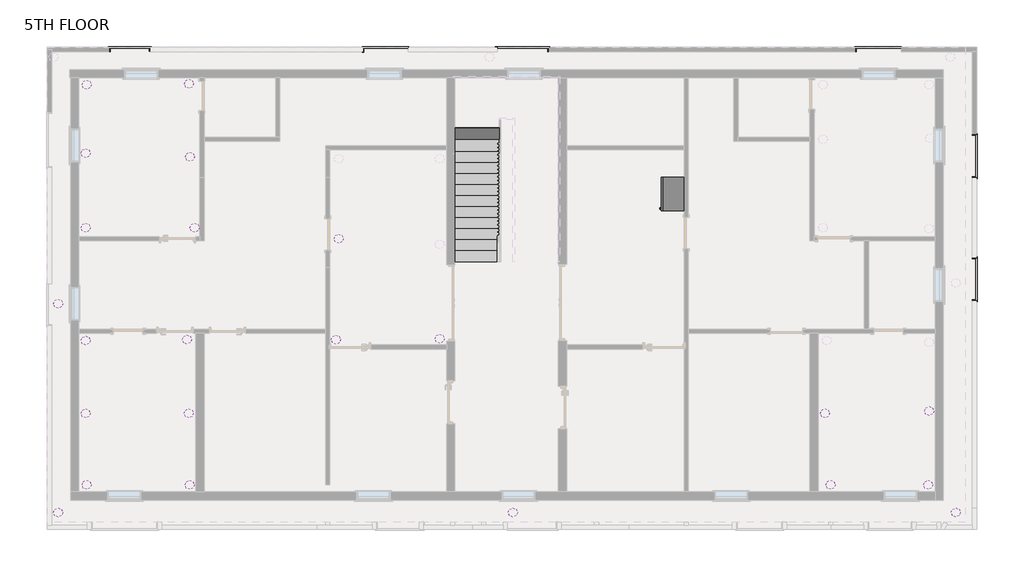
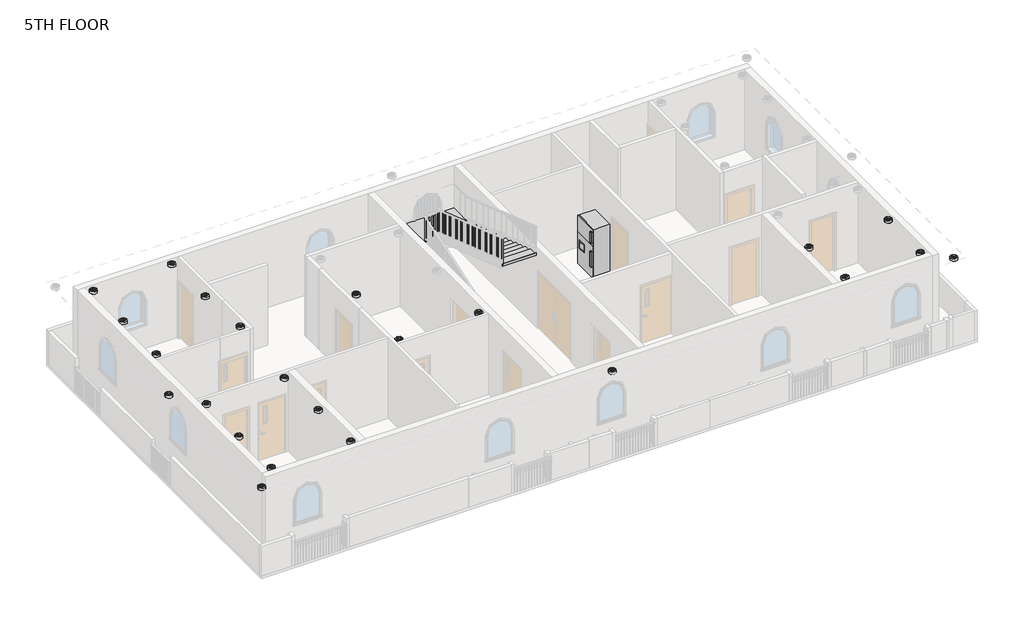
# One storey, part 6 of 7: 23 light fixtures, 6 railings, 1 furniture element, 1 stair flight.
# Revit data of these elements (continued)
# Element 21 (IfcLightFixture, "Ceiling Light - Flat Round : 60W - 120V") (continued)
#   Materials on its faces: "Glass, White, High Luminance", "Steel, Paint Finish, Dark Gray, Matte"
# Element 22 (IfcLightFixture, "Ceiling Light - Flat Round : 60W - 120V")
#   Mark = "171"
#   built-in parameter 1140040 = 1
#   Phase Created = New Construction
#   Materials on its faces: "Glass, White, High Luminance", "Steel, Paint Finish, Dark Gray, Matte"
# Element 23 (IfcLightFixture, "Ceiling Light - Flat Round : 60W - 120V")
#   Mark = "172"
#   built-in parameter 1140040 = 1
#   Phase Created = New Construction
#   Materials on its faces: "Glass, White, High Luminance", "Steel, Paint Finish, Dark Gray, Matte"
# Element 24 (IfcLightFixture, "Ceiling Light - Flat Round : 60W - 120V")
#   Mark = "173"
#   built-in parameter 1140040 = 1
#   Phase Created = New Construction
#   Materials on its faces: "Glass, White, High Luminance", "Steel, Paint Finish, Dark Gray, Matte"
# Elements 25, 26, 27, 28, 29, 30 (IfcRailing, "Handrail - Rectangular")
#   Phase Created = New Construction
# Element 31 (IfcStairFlight, "2\" Tread 1\" Nosing 1/4\" Riser")
#   Phase Created = New Construction
# Materials
#   "Steel, Paint Finish, Dark Gray, Matte": class "Metal", colour RGB 98 98 98, transparency 0, Description = "Steel, paint finish, dark gray, matte", Cost = 0
#   "Glass, White, High Luminance": class "Glass", colour RGB 249 250 249, transparency 0.8, Description = "physical material", Cost = 0
#   "Default": colour RGB 127 127 127, transparency 0, Cost = 0
#   "Default 3": class "Glass", colour RGB 127 127 127, transparency 0
#   "Default 2": class "Plastic", colour RGB 127 127 127, transparency 0
